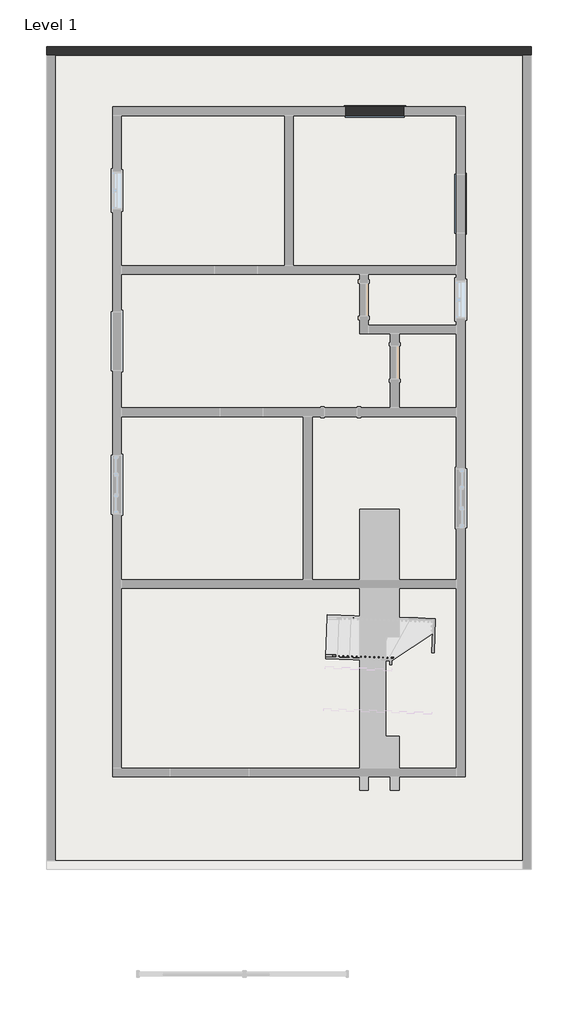
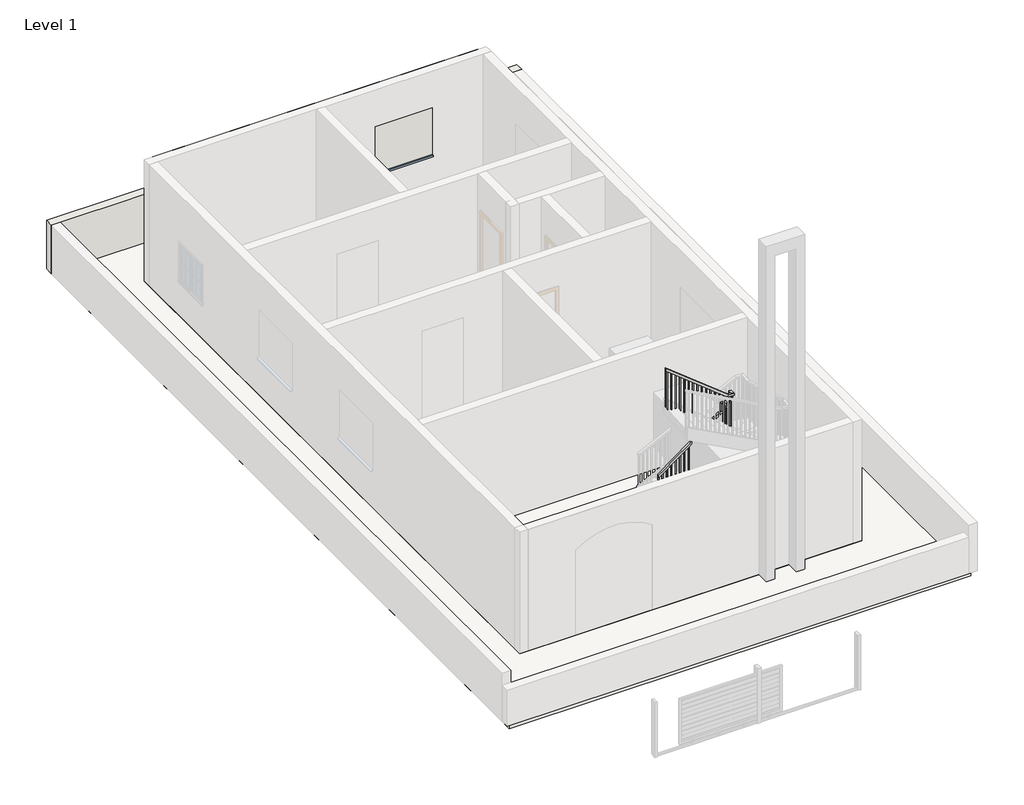
# One storey, part 2 of 4: 3 slabs, 2 railings, 2 walls, 2 windows.
"""IFC4 building model written with IfcOpenShell, lengths in millimetres."""

from ifc_helpers import new_model, si_unit, frame, origin, place, context, project, spatial, polyline, outline, extrude, faceted_brep, transform, mapped, element, save
from components import windows_tpl_plain_1360x1210mm_e2a6c9d8

model = new_model("IFC4")

# Units and contexts
model_context = context("Model", 3, world=origin())
ifc_project = project(units=[si_unit("LENGTHUNIT", "METRE", prefix="MILLI")], contexts=[model_context])

# Site, building, storey
site = spatial("IfcSite", under=ifc_project)
building = spatial("IfcBuilding", under=site)
storey = spatial("IfcBuildingStorey", under=building, Name="Level 1", Elevation=0.0)

# Railings
placement = place(None, origin())
element("IfcRailing", 1, ObjectType="Handrail - Rectangular", at=placement, inside=storey, context=model_context, shape_type="SolidModel", body=[
    faceted_brep([(-10037.4477622, -1226.3543786, 1083.7333333), (-10037.4477622, -1226.3543786, 1019.4000346), (-10039.2744432, -1277.1215258, 1019.4000346), (-10039.2744432, -1277.1215258, 1083.7333333), (-8586.854788, -1278.5489726, 2211.6191036), (-8536.0876408, -1280.3756536, 2186.7590024), (-8537.9143218, -1331.1428009, 2186.7590024), (-8588.681469, -1329.3161198, 2211.6191036), (-8586.854788, -1278.5489726, 2414.6281882), (-8536.0876408, -1280.3756536, 2363.8281882), (-8537.9143218, -1331.1428009, 2363.8281882), (-8588.681469, -1329.3161198, 2414.6281882), (-8459.9369199, -1283.1156752, 2414.6281882), (-8459.9369199, -1283.1156752, 2363.8281882), (-8512.5307482, -1332.0561414, 2363.8281882), (-8512.5307482, -1332.0561414, 2414.6281882), (-8464.5036225, -1410.0335432, 2414.6281882), (-8465.5507758, -1439.136044, 2363.8281882), (-8516.317923, -1437.309363, 2363.8281882), (-8515.2707697, -1408.2068622, 2414.6281882), (-8469.070325, -1536.9514112, 2631.5051451), (-8470.897006, -1587.7185585, 2617.7256424), (-8521.6641532, -1585.8918774, 2617.7256424), (-8519.8374722, -1535.1247302, 2631.5051451), (-8469.070325, -1536.9514112, 2834.5142297), (-8470.897006, -1587.7185585, 2783.7142297), (-8521.6641532, -1585.8918774, 2783.7142297), (-8519.8374722, -1535.1247302, 2834.5142297), (-8473.6370275, -1663.8692793, 2834.5142297), (-8473.6370275, -1663.8692793, 2783.7142297), (-8522.5774937, -1611.2754511, 2783.7142297), (-8522.5774937, -1611.2754511, 2834.5142297), (-8600.5548956, -1659.3025768, 2834.5142297), (-8617.9603, -1658.6763032, 2783.7142297), (-8616.133619, -1607.909156, 2783.7142297), (-8598.7282145, -1608.5354295, 2834.5142297), (-10051.1478698, -1607.1079827, 3962.4), (-10049.3211887, -1556.3408355, 3962.4), (-10049.3211887, -1556.3408355, 3898.0667013), (-10051.1478698, -1607.1079827, 3898.0667013)], [[[0, 1, 2, 3]], [[1, 0, 4, 5]], [[2, 1, 5, 6]], [[3, 2, 6, 7]], [[0, 3, 7, 4]], [[5, 4, 8, 9]], [[6, 5, 9, 10]], [[7, 6, 10, 11]], [[4, 7, 11, 8]], [[9, 8, 12, 13]], [[10, 9, 13, 14]], [[11, 10, 14, 15]], [[8, 11, 15, 12]], [[13, 12, 16, 17]], [[14, 13, 17, 18]], [[15, 14, 18, 19]], [[12, 15, 19, 16]], [[17, 16, 20, 21]], [[18, 17, 21, 22]], [[19, 18, 22, 23]], [[16, 19, 23, 20]], [[21, 20, 24, 25]], [[22, 21, 25, 26]], [[23, 22, 26, 27]], [[20, 23, 27, 24]], [[25, 24, 28, 29]], [[26, 25, 29, 30]], [[27, 26, 30, 31]], [[24, 27, 31, 28]], [[29, 28, 32, 33]], [[30, 29, 33, 34]], [[31, 30, 34, 35]], [[28, 31, 35, 32]], [[36, 37, 38, 39]], [[33, 32, 36, 39]], [[34, 33, 39, 38]], [[35, 34, 38, 37]], [[32, 35, 37, 36]]]),
    extrude(outline(polyline([(236.0012245, -19.05), (221.1987754, 0.0), (1225.3637939, 0.0), (1225.3637939, -19.05), (236.0012245, -19.05)])), frame((-10030.9830199, -1591.9482723, 4104.0304606), z_axis=(0.0359582876180528, 0.9993532916599503, 0.0), x_axis=(0.0, 0.0, -1.0)), (0.0, 0.0, 1.0), 19.05),
    extrude(outline(polyline([(236.0012246, -19.05), (221.1987755, 0.0), (1146.417399, 0.0), (1146.417399, -19.05), (236.0012246, -19.05)])), frame((-9929.4487255, -1595.6016343, 4025.0840657), z_axis=(0.0359582876180528, 0.9993532916599503, 0.0), x_axis=(0.0, 0.0, -1.0)), (0.0, 0.0, 1.0), 19.05),
    extrude(outline(polyline([(236.0012245, -19.05), (221.1987755, 0.0), (1067.471004, 0.0), (1067.471004, -19.05), (236.0012245, -19.05)])), frame((-9827.914431, -1599.2549963, 3946.1376707), z_axis=(0.0359582876180528, 0.9993532916599503, 0.0), x_axis=(0.0, 0.0, -1.0)), (0.0, 0.0, 1.0), 19.05),
    extrude(outline(polyline([(236.0012245, -19.05), (221.1987754, 0.0), (1157.8579424, 0.0), (1157.8579424, -19.05), (236.0012245, -19.05)])), frame((-9726.3801366, -1602.9083583, 3867.1912757), z_axis=(0.0359582876180528, 0.9993532916599503, 0.0), x_axis=(0.0, 0.0, -1.0)), (0.0, 0.0, 1.0), 19.05),
    extrude(outline(polyline([(236.0012246, -19.05), (221.1987755, 0.0), (1078.9115475, 0.0), (1078.9115475, -19.05), (236.0012246, -19.05)])), frame((-9624.8458422, -1606.5617203, 3788.2448808), z_axis=(0.0359582876180528, 0.9993532916599503, 0.0), x_axis=(0.0, 0.0, -1.0)), (0.0, 0.0, 1.0), 19.05),
    extrude(outline(polyline([(236.0012245, -19.05), (221.1987755, 0.0), (999.9651525, 0.0), (999.9651525, -19.05), (236.0012245, -19.05)])), frame((-9523.3115477, -1610.2150824, 3709.2984858), z_axis=(0.0359582876180528, 0.9993532916599503, 0.0), x_axis=(0.0, 0.0, -1.0)), (0.0, 0.0, 1.0), 19.05),
    extrude(outline(polyline([(236.0012245, -19.05), (221.1987754, 0.0), (1090.3520908, 0.0), (1090.3520908, -19.05), (236.0012245, -19.05)])), frame((-9421.7772533, -1613.8684444, 3630.3520908), z_axis=(0.0359582876180528, 0.9993532916599503, 0.0), x_axis=(0.0, 0.0, -1.0)), (0.0, 0.0, 1.0), 19.05),
    extrude(outline(polyline([(236.0012246, -19.05), (221.1987755, 0.0), (1011.4056959, 0.0), (1011.4056959, -19.05), (236.0012246, -19.05)])), frame((-9320.2429589, -1617.5218064, 3551.4056959), z_axis=(0.0359582876180528, 0.9993532916599503, 0.0), x_axis=(0.0, 0.0, -1.0)), (0.0, 0.0, 1.0), 19.05),
    extrude(outline(polyline([(236.0012245, -19.05), (221.1987755, 0.0), (1101.7926342, 0.0), (1101.7926342, -19.05), (236.0012245, -19.05)])), frame((-9218.7086644, -1621.1751684, 3472.4593009), z_axis=(0.0359582876180528, 0.9993532916599503, 0.0), x_axis=(0.0, 0.0, -1.0)), (0.0, 0.0, 1.0), 19.05),
    extrude(outline(polyline([(236.0012245, -19.05), (221.1987755, 0.0), (1022.8462392, 0.0), (1022.8462392, -19.05), (236.0012245, -19.05)])), frame((-9117.17437, -1624.8285304, 3393.5129059), z_axis=(0.0359582876180528, 0.9993532916599503, 0.0), x_axis=(0.0, 0.0, -1.0)), (0.0, 0.0, 1.0), 19.05),
    extrude(outline(polyline([(236.0012245, -19.05), (221.1987754, 0.0), (943.8998442, 0.0), (943.8998442, -19.05), (236.0012245, -19.05)])), frame((-9015.6400756, -1628.4818925, 3314.5665109), z_axis=(0.0359582876180528, 0.9993532916599503, 0.0), x_axis=(0.0, 0.0, -1.0)), (0.0, 0.0, 1.0), 19.05),
    extrude(outline(polyline([(236.0012246, -19.05), (221.1987755, 0.0), (1034.2867827, 0.0), (1034.2867827, -19.05), (236.0012246, -19.05)])), frame((-8914.1057811, -1632.1352545, 3235.620116), z_axis=(0.0359582876180528, 0.9993532916599503, 0.0), x_axis=(0.0, 0.0, -1.0)), (0.0, 0.0, 1.0), 19.05),
    extrude(outline(polyline([(236.0012245, -19.05), (221.1987755, 0.0), (955.3403877, 0.0), (955.3403877, -19.05), (236.0012245, -19.05)])), frame((-8812.5714867, -1635.7886165, 3156.673721), z_axis=(0.0359582876180528, 0.9993532916599503, 0.0), x_axis=(0.0, 0.0, -1.0)), (0.0, 0.0, 1.0), 19.05),
    extrude(outline(polyline([(236.0012245, -19.05), (221.1987754, 0.0), (1045.727326, 0.0), (1045.727326, -19.05), (236.0012245, -19.05)])), frame((-8711.0371923, -1639.4419785, 3077.727326), z_axis=(0.0359582876180528, 0.9993532916599503, 0.0), x_axis=(0.0, 0.0, -1.0)), (0.0, 0.0, 1.0), 19.05),
    extrude(outline(polyline([(236.0012246, -19.05), (221.1987755, 0.0), (966.7809311, 0.0), (966.7809311, -19.05), (236.0012246, -19.05)])), frame((-8609.5028978, -1643.0953406, 2998.7809311), z_axis=(0.0359582876180528, 0.9993532916599503, 0.0), x_axis=(0.0, 0.0, -1.0)), (0.0, 0.0, 1.0), 19.05),
    extrude(outline(polyline([(-8506.3702575, -1602.3274488), (-8487.3325773, -1603.0124541), (-8488.0175827, -1622.0501344), (-8507.0552629, -1621.365129), (-8506.3702575, -1602.3274488)])), frame((0.0, 0.0, 1693.3333333), z_axis=(0.0, 0.0, 1.0), x_axis=(1.0, 0.0, 0.0)), (0.0, 0.0, 1.0), 1090.3808964),
    extrude(outline(polyline([(244.8657718, -19.05), (212.3342282, 0.0), (1192.1994682, 0.0), (1192.1994682, -19.05), (244.8657718, -19.05)])), frame((-8484.3642207, -1520.5158399, 2716.1994682), z_axis=(-0.9993532916599502, 0.035958287618050686, 0.0), x_axis=(0.0, 0.0, -1.0)), (0.0, 0.0, 1.0), 19.05),
    extrude(outline(polyline([(244.8657717, -19.05), (212.3342282, 0.0), (1188.0312359, 0.0), (1188.0312359, -19.05), (244.8657717, -19.05)])), frame((-8480.7108586, -1418.9815455, 2542.6979026), z_axis=(-0.9993532916599502, 0.035958287618050686, 0.0), x_axis=(0.0, 0.0, -1.0)), (0.0, 0.0, 1.0), 19.05),
    extrude(outline(polyline([(-8525.208029, -1315.7147199), (-8524.5230236, -1296.6770397), (-8505.4853434, -1297.3620451), (-8506.1703488, -1316.3997253), (-8525.208029, -1315.7147199)])), frame((0.0, 0.0, 1185.3333333), z_axis=(0.0, 0.0, 1.0), x_axis=(1.0, 0.0, 0.0)), (0.0, 0.0, 1.0), 1178.4948549),
    extrude(outline(polyline([(221.1987754, -19.05), (236.0012245, 0.0), (1337.2495642, 0.0), (1337.2495642, -19.05), (221.1987754, -19.05)])), frame((-8626.7423234, -1312.0613579, 2353.2495642), z_axis=(0.035958287618052934, 0.9993532916599503, 0.0), x_axis=(0.0, 0.0, -1.0)), (0.0, 0.0, 1.0), 19.05),
    extrude(outline(polyline([(221.1987755, -19.0500001), (236.0012246, 0.0), (1258.3031693, 0.0), (1258.3031693, -19.0500001), (221.1987755, -19.0500001)])), frame((-8728.2766179, -1308.4079959, 2274.3031693), z_axis=(0.035958287618052934, 0.9993532916599503, 0.0), x_axis=(0.0, 0.0, -1.0)), (0.0, 0.0, 1.0), 19.05),
    extrude(outline(polyline([(221.1987755, -19.05), (236.0012245, 0.0), (1348.6901076, 0.0), (1348.6901076, -19.05), (221.1987755, -19.05)])), frame((-8829.8109123, -1304.7546339, 2195.3567743), z_axis=(0.035958287618052934, 0.9993532916599503, 0.0), x_axis=(0.0, 0.0, -1.0)), (0.0, 0.0, 1.0), 19.05),
    extrude(outline(polyline([(221.1987754, -19.05), (236.0012245, 0.0), (1269.7437126, 0.0), (1269.7437126, -19.05), (221.1987754, -19.05)])), frame((-8931.3452067, -1301.1012718, 2116.4103793), z_axis=(0.035958287618052934, 0.9993532916599503, 0.0), x_axis=(0.0, 0.0, -1.0)), (0.0, 0.0, 1.0), 19.05),
    extrude(outline(polyline([(221.1987755, -19.05), (236.0012246, 0.0), (1360.1306511, 0.0), (1360.1306511, -19.05), (221.1987755, -19.05)])), frame((-9032.8795011, -1297.4479098, 2037.4639844), z_axis=(0.035958287618052934, 0.9993532916599503, 0.0), x_axis=(0.0, 0.0, -1.0)), (0.0, 0.0, 1.0), 19.05),
    extrude(outline(polyline([(221.1987755, -19.05), (236.0012245, 0.0), (1281.1842561, 0.0), (1281.1842561, -19.05), (221.1987755, -19.05)])), frame((-9134.4137956, -1293.7945478, 1958.5175894), z_axis=(0.035958287618052934, 0.9993532916599503, 0.0), x_axis=(0.0, 0.0, -1.0)), (0.0, 0.0, 1.0), 19.05),
    extrude(outline(polyline([(221.1987755, -19.05), (236.0012245, 0.0), (1371.5711944, 0.0), (1371.5711944, -19.05), (221.1987755, -19.05)])), frame((-9235.94809, -1290.1411858, 1879.5711944), z_axis=(0.035958287618052934, 0.9993532916599503, 0.0), x_axis=(0.0, 0.0, -1.0)), (0.0, 0.0, 1.0), 19.05),
    extrude(outline(polyline([(221.1987754, -19.05), (236.0012245, 0.0), (1292.6247994, 0.0), (1292.6247994, -19.05), (221.1987754, -19.05)])), frame((-9337.4823844, -1286.4878237, 1800.6247994), z_axis=(0.035958287618052934, 0.9993532916599503, 0.0), x_axis=(0.0, 0.0, -1.0)), (0.0, 0.0, 1.0), 19.05),
    extrude(outline(polyline([(221.1987755, -19.05), (236.0012246, 0.0), (1213.6784045, 0.0), (1213.6784045, -19.05), (221.1987755, -19.05)])), frame((-9439.0166789, -1282.8344617, 1721.6784045), z_axis=(0.035958287618052934, 0.9993532916599503, 0.0), x_axis=(0.0, 0.0, -1.0)), (0.0, 0.0, 1.0), 19.05),
    extrude(outline(polyline([(221.1987755, -19.05), (236.0012245, 0.0), (1304.0653428, 0.0), (1304.0653428, -19.05), (221.1987755, -19.05)])), frame((-9540.5509733, -1279.1810997, 1642.7320095), z_axis=(0.035958287618052934, 0.9993532916599503, 0.0), x_axis=(0.0, 0.0, -1.0)), (0.0, 0.0, 1.0), 19.05),
    extrude(outline(polyline([(221.1987754, -19.05), (236.0012245, 0.0), (1225.1189478, 0.0), (1225.1189478, -19.05), (221.1987754, -19.05)])), frame((-9642.0852677, -1275.5277377, 1563.7856145), z_axis=(0.035958287618052934, 0.9993532916599503, 0.0), x_axis=(0.0, 0.0, -1.0)), (0.0, 0.0, 1.0), 19.05),
    extrude(outline(polyline([(221.1987755, -19.05), (236.0012246, 0.0), (1146.1725529, 0.0), (1146.1725529, -19.05), (221.1987755, -19.05)])), frame((-9743.6195622, -1271.8743757, 1484.8392196), z_axis=(0.035958287618052934, 0.9993532916599503, 0.0), x_axis=(0.0, 0.0, -1.0)), (0.0, 0.0, 1.0), 19.05),
    extrude(outline(polyline([(221.1987755, -19.05), (236.0012245, 0.0), (1236.5594913, 0.0), (1236.5594913, -19.05), (221.1987755, -19.05)])), frame((-9845.1538566, -1268.2210136, 1405.8928246), z_axis=(0.035958287618052934, 0.9993532916599503, 0.0), x_axis=(0.0, 0.0, -1.0)), (0.0, 0.0, 1.0), 19.05),
    extrude(outline(polyline([(221.1987755, -19.05), (236.0012245, 0.0), (1157.6130963, 0.0), (1157.6130963, -19.05), (221.1987755, -19.05)])), frame((-9946.688151, -1264.5676516, 1326.9464296), z_axis=(0.035958287618052934, 0.9993532916599503, 0.0), x_axis=(0.0, 0.0, -1.0)), (0.0, 0.0, 1.0), 19.05),
    extrude(outline(polyline([(-8507.283598, -1627.7110224), (-8488.2459178, -1628.3960278), (-8488.9309232, -1647.433708), (-8507.9686034, -1646.7487026), (-8507.283598, -1627.7110224)])), frame((0.0, 0.0, 1862.6666667), z_axis=(0.0, 0.0, 1.0), x_axis=(1.0, 0.0, 0.0)), (0.0, 0.0, 1.0), 921.0475631),
    extrude(outline(polyline([(-8496.0951768, -1316.7622457), (-8495.4101715, -1297.7245655), (-8476.3724912, -1298.4095708), (-8477.0574966, -1317.4472511), (-8496.0951768, -1316.7622457)])), frame((0.0, 0.0, 1185.3333333), z_axis=(0.0, 0.0, 1.0), x_axis=(1.0, 0.0, 0.0)), (0.0, 0.0, 1.0), 1178.4948549),
    extrude(outline(polyline([(236.0012245, -19.05), (221.1987755, 0.0), (1240.5988101, 0.0), (1240.5988101, -19.05), (236.0012245, -19.05)])), frame((-10050.5770319, -1591.2432492, 4119.2654768), z_axis=(0.0359582876180528, 0.9993532916599503, 0.0), x_axis=(0.0, 0.0, -1.0)), (0.0, 0.0, 1.0), 19.05),
    extrude(outline(polyline([(221.1987755, -19.05), (236.0012246, 0.0), (1086.0679259, 0.0), (1086.0679259, -19.05), (221.1987755, -19.05)])), frame((-10038.7036054, -1261.2567923, 1255.4012592), z_axis=(0.035958287618052934, 0.9993532916599503, 0.0), x_axis=(0.0, 0.0, -1.0)), (0.0, 0.0, 1.0), 19.05),
])
element("IfcRailing", 2, ObjectType="Handrail - Rectangular", at=placement, inside=storey, context=model_context, shape_type="SolidModel", body=[
    faceted_brep([(-10037.4477622, -1226.3543786, 1083.7333333), (-10037.4477622, -1226.3543786, 1019.4000346), (-10039.2744432, -1277.1215258, 1019.4000346), (-10039.2744432, -1277.1215258, 1083.7333333), (-8586.854788, -1278.5489726, 2211.6191036), (-8536.0876408, -1280.3756536, 2186.7590024), (-8537.9143218, -1331.1428009, 2186.7590024), (-8588.681469, -1329.3161198, 2211.6191036), (-8586.854788, -1278.5489726, 2414.6281882), (-8536.0876408, -1280.3756536, 2363.8281882), (-8537.9143218, -1331.1428009, 2363.8281882), (-8588.681469, -1329.3161198, 2414.6281882), (-8459.9369199, -1283.1156752, 2414.6281882), (-8459.9369199, -1283.1156752, 2363.8281882), (-8512.5307482, -1332.0561414, 2363.8281882), (-8512.5307482, -1332.0561414, 2414.6281882), (-8464.5036225, -1410.0335432, 2414.6281882), (-8465.5507758, -1439.136044, 2363.8281882), (-8516.317923, -1437.309363, 2363.8281882), (-8515.2707697, -1408.2068622, 2414.6281882), (-8469.070325, -1536.9514112, 2631.5051451), (-8470.897006, -1587.7185585, 2617.7256424), (-8521.6641532, -1585.8918774, 2617.7256424), (-8519.8374722, -1535.1247302, 2631.5051451), (-8469.070325, -1536.9514112, 2834.5142297), (-8470.897006, -1587.7185585, 2783.7142297), (-8521.6641532, -1585.8918774, 2783.7142297), (-8519.8374722, -1535.1247302, 2834.5142297), (-8473.6370275, -1663.8692793, 2834.5142297), (-8473.6370275, -1663.8692793, 2783.7142297), (-8522.5774937, -1611.2754511, 2783.7142297), (-8522.5774937, -1611.2754511, 2834.5142297), (-8600.5548956, -1659.3025768, 2834.5142297), (-8617.9603, -1658.6763032, 2783.7142297), (-8616.133619, -1607.909156, 2783.7142297), (-8598.7282145, -1608.5354295, 2834.5142297), (-10051.1478698, -1607.1079827, 3962.4), (-10049.3211887, -1556.3408355, 3962.4), (-10049.3211887, -1556.3408355, 3898.0667013), (-10051.1478698, -1607.1079827, 3898.0667013)], [[[0, 1, 2, 3]], [[1, 0, 4, 5]], [[2, 1, 5, 6]], [[3, 2, 6, 7]], [[0, 3, 7, 4]], [[5, 4, 8, 9]], [[6, 5, 9, 10]], [[7, 6, 10, 11]], [[4, 7, 11, 8]], [[9, 8, 12, 13]], [[10, 9, 13, 14]], [[11, 10, 14, 15]], [[8, 11, 15, 12]], [[13, 12, 16, 17]], [[14, 13, 17, 18]], [[15, 14, 18, 19]], [[12, 15, 19, 16]], [[17, 16, 20, 21]], [[18, 17, 21, 22]], [[19, 18, 22, 23]], [[16, 19, 23, 20]], [[21, 20, 24, 25]], [[22, 21, 25, 26]], [[23, 22, 26, 27]], [[20, 23, 27, 24]], [[25, 24, 28, 29]], [[26, 25, 29, 30]], [[27, 26, 30, 31]], [[24, 27, 31, 28]], [[29, 28, 32, 33]], [[30, 29, 33, 34]], [[31, 30, 34, 35]], [[28, 31, 35, 32]], [[36, 37, 38, 39]], [[33, 32, 36, 39]], [[34, 33, 39, 38]], [[35, 34, 38, 37]], [[32, 35, 37, 36]]]),
    extrude(outline(polyline([(236.0012245, -19.05), (221.1987754, 0.0), (1225.3637939, 0.0), (1225.3637939, -19.05), (236.0012245, -19.05)])), frame((-10030.9830199, -1591.9482723, 4104.0304606), z_axis=(0.0359582876180528, 0.9993532916599503, 0.0), x_axis=(0.0, 0.0, -1.0)), (0.0, 0.0, 1.0), 19.05),
    extrude(outline(polyline([(236.0012246, -19.05), (221.1987755, 0.0), (1146.417399, 0.0), (1146.417399, -19.05), (236.0012246, -19.05)])), frame((-9929.4487255, -1595.6016343, 4025.0840657), z_axis=(0.0359582876180528, 0.9993532916599503, 0.0), x_axis=(0.0, 0.0, -1.0)), (0.0, 0.0, 1.0), 19.05),
    extrude(outline(polyline([(236.0012245, -19.05), (221.1987755, 0.0), (1067.471004, 0.0), (1067.471004, -19.05), (236.0012245, -19.05)])), frame((-9827.914431, -1599.2549963, 3946.1376707), z_axis=(0.0359582876180528, 0.9993532916599503, 0.0), x_axis=(0.0, 0.0, -1.0)), (0.0, 0.0, 1.0), 19.05),
    extrude(outline(polyline([(236.0012245, -19.05), (221.1987754, 0.0), (1157.8579424, 0.0), (1157.8579424, -19.05), (236.0012245, -19.05)])), frame((-9726.3801366, -1602.9083583, 3867.1912757), z_axis=(0.0359582876180528, 0.9993532916599503, 0.0), x_axis=(0.0, 0.0, -1.0)), (0.0, 0.0, 1.0), 19.05),
    extrude(outline(polyline([(236.0012246, -19.05), (221.1987755, 0.0), (1078.9115475, 0.0), (1078.9115475, -19.05), (236.0012246, -19.05)])), frame((-9624.8458422, -1606.5617203, 3788.2448808), z_axis=(0.0359582876180528, 0.9993532916599503, 0.0), x_axis=(0.0, 0.0, -1.0)), (0.0, 0.0, 1.0), 19.05),
    extrude(outline(polyline([(236.0012245, -19.05), (221.1987755, 0.0), (999.9651525, 0.0), (999.9651525, -19.05), (236.0012245, -19.05)])), frame((-9523.3115477, -1610.2150824, 3709.2984858), z_axis=(0.0359582876180528, 0.9993532916599503, 0.0), x_axis=(0.0, 0.0, -1.0)), (0.0, 0.0, 1.0), 19.05),
    extrude(outline(polyline([(236.0012245, -19.05), (221.1987754, 0.0), (1090.3520908, 0.0), (1090.3520908, -19.05), (236.0012245, -19.05)])), frame((-9421.7772533, -1613.8684444, 3630.3520908), z_axis=(0.0359582876180528, 0.9993532916599503, 0.0), x_axis=(0.0, 0.0, -1.0)), (0.0, 0.0, 1.0), 19.05),
    extrude(outline(polyline([(236.0012246, -19.05), (221.1987755, 0.0), (1011.4056959, 0.0), (1011.4056959, -19.05), (236.0012246, -19.05)])), frame((-9320.2429589, -1617.5218064, 3551.4056959), z_axis=(0.0359582876180528, 0.9993532916599503, 0.0), x_axis=(0.0, 0.0, -1.0)), (0.0, 0.0, 1.0), 19.05),
    extrude(outline(polyline([(236.0012245, -19.05), (221.1987755, 0.0), (1101.7926342, 0.0), (1101.7926342, -19.05), (236.0012245, -19.05)])), frame((-9218.7086644, -1621.1751684, 3472.4593009), z_axis=(0.0359582876180528, 0.9993532916599503, 0.0), x_axis=(0.0, 0.0, -1.0)), (0.0, 0.0, 1.0), 19.05),
    extrude(outline(polyline([(236.0012245, -19.05), (221.1987755, 0.0), (1022.8462392, 0.0), (1022.8462392, -19.05), (236.0012245, -19.05)])), frame((-9117.17437, -1624.8285304, 3393.5129059), z_axis=(0.0359582876180528, 0.9993532916599503, 0.0), x_axis=(0.0, 0.0, -1.0)), (0.0, 0.0, 1.0), 19.05),
    extrude(outline(polyline([(236.0012245, -19.05), (221.1987754, 0.0), (943.8998442, 0.0), (943.8998442, -19.05), (236.0012245, -19.05)])), frame((-9015.6400756, -1628.4818925, 3314.5665109), z_axis=(0.0359582876180528, 0.9993532916599503, 0.0), x_axis=(0.0, 0.0, -1.0)), (0.0, 0.0, 1.0), 19.05),
    extrude(outline(polyline([(236.0012246, -19.05), (221.1987755, 0.0), (1034.2867827, 0.0), (1034.2867827, -19.05), (236.0012246, -19.05)])), frame((-8914.1057811, -1632.1352545, 3235.620116), z_axis=(0.0359582876180528, 0.9993532916599503, 0.0), x_axis=(0.0, 0.0, -1.0)), (0.0, 0.0, 1.0), 19.05),
    extrude(outline(polyline([(236.0012245, -19.05), (221.1987755, 0.0), (955.3403877, 0.0), (955.3403877, -19.05), (236.0012245, -19.05)])), frame((-8812.5714867, -1635.7886165, 3156.673721), z_axis=(0.0359582876180528, 0.9993532916599503, 0.0), x_axis=(0.0, 0.0, -1.0)), (0.0, 0.0, 1.0), 19.05),
    extrude(outline(polyline([(236.0012245, -19.05), (221.1987754, 0.0), (1045.727326, 0.0), (1045.727326, -19.05), (236.0012245, -19.05)])), frame((-8711.0371923, -1639.4419785, 3077.727326), z_axis=(0.0359582876180528, 0.9993532916599503, 0.0), x_axis=(0.0, 0.0, -1.0)), (0.0, 0.0, 1.0), 19.05),
    extrude(outline(polyline([(236.0012246, -19.05), (221.1987755, 0.0), (966.7809311, 0.0), (966.7809311, -19.05), (236.0012246, -19.05)])), frame((-8609.5028978, -1643.0953406, 2998.7809311), z_axis=(0.0359582876180528, 0.9993532916599503, 0.0), x_axis=(0.0, 0.0, -1.0)), (0.0, 0.0, 1.0), 19.05),
    extrude(outline(polyline([(-8506.3702575, -1602.3274488), (-8487.3325773, -1603.0124541), (-8488.0175827, -1622.0501344), (-8507.0552629, -1621.365129), (-8506.3702575, -1602.3274488)])), frame((0.0, 0.0, 1693.3333333), z_axis=(0.0, 0.0, 1.0), x_axis=(1.0, 0.0, 0.0)), (0.0, 0.0, 1.0), 1090.3808964),
    extrude(outline(polyline([(244.8657718, -19.05), (212.3342282, 0.0), (1192.1994682, 0.0), (1192.1994682, -19.05), (244.8657718, -19.05)])), frame((-8484.3642207, -1520.5158399, 2716.1994682), z_axis=(-0.9993532916599502, 0.035958287618050686, 0.0), x_axis=(0.0, 0.0, -1.0)), (0.0, 0.0, 1.0), 19.05),
    extrude(outline(polyline([(244.8657717, -19.05), (212.3342282, 0.0), (1188.0312359, 0.0), (1188.0312359, -19.05), (244.8657717, -19.05)])), frame((-8480.7108586, -1418.9815455, 2542.6979026), z_axis=(-0.9993532916599502, 0.035958287618050686, 0.0), x_axis=(0.0, 0.0, -1.0)), (0.0, 0.0, 1.0), 19.05),
    extrude(outline(polyline([(-8525.208029, -1315.7147199), (-8524.5230236, -1296.6770397), (-8505.4853434, -1297.3620451), (-8506.1703488, -1316.3997253), (-8525.208029, -1315.7147199)])), frame((0.0, 0.0, 1185.3333333), z_axis=(0.0, 0.0, 1.0), x_axis=(1.0, 0.0, 0.0)), (0.0, 0.0, 1.0), 1178.4948549),
    extrude(outline(polyline([(221.1987754, -19.05), (236.0012245, 0.0), (1337.2495642, 0.0), (1337.2495642, -19.05), (221.1987754, -19.05)])), frame((-8626.7423234, -1312.0613579, 2353.2495642), z_axis=(0.035958287618052934, 0.9993532916599503, 0.0), x_axis=(0.0, 0.0, -1.0)), (0.0, 0.0, 1.0), 19.05),
    extrude(outline(polyline([(221.1987755, -19.0500001), (236.0012246, 0.0), (1258.3031693, 0.0), (1258.3031693, -19.0500001), (221.1987755, -19.0500001)])), frame((-8728.2766179, -1308.4079959, 2274.3031693), z_axis=(0.035958287618052934, 0.9993532916599503, 0.0), x_axis=(0.0, 0.0, -1.0)), (0.0, 0.0, 1.0), 19.05),
    extrude(outline(polyline([(221.1987755, -19.05), (236.0012245, 0.0), (1348.6901076, 0.0), (1348.6901076, -19.05), (221.1987755, -19.05)])), frame((-8829.8109123, -1304.7546339, 2195.3567743), z_axis=(0.035958287618052934, 0.9993532916599503, 0.0), x_axis=(0.0, 0.0, -1.0)), (0.0, 0.0, 1.0), 19.05),
    extrude(outline(polyline([(221.1987754, -19.05), (236.0012245, 0.0), (1269.7437126, 0.0), (1269.7437126, -19.05), (221.1987754, -19.05)])), frame((-8931.3452067, -1301.1012718, 2116.4103793), z_axis=(0.035958287618052934, 0.9993532916599503, 0.0), x_axis=(0.0, 0.0, -1.0)), (0.0, 0.0, 1.0), 19.05),
    extrude(outline(polyline([(221.1987755, -19.05), (236.0012246, 0.0), (1360.1306511, 0.0), (1360.1306511, -19.05), (221.1987755, -19.05)])), frame((-9032.8795011, -1297.4479098, 2037.4639844), z_axis=(0.035958287618052934, 0.9993532916599503, 0.0), x_axis=(0.0, 0.0, -1.0)), (0.0, 0.0, 1.0), 19.05),
    extrude(outline(polyline([(221.1987755, -19.05), (236.0012245, 0.0), (1281.1842561, 0.0), (1281.1842561, -19.05), (221.1987755, -19.05)])), frame((-9134.4137956, -1293.7945478, 1958.5175894), z_axis=(0.035958287618052934, 0.9993532916599503, 0.0), x_axis=(0.0, 0.0, -1.0)), (0.0, 0.0, 1.0), 19.05),
    extrude(outline(polyline([(221.1987755, -19.05), (236.0012245, 0.0), (1371.5711944, 0.0), (1371.5711944, -19.05), (221.1987755, -19.05)])), frame((-9235.94809, -1290.1411858, 1879.5711944), z_axis=(0.035958287618052934, 0.9993532916599503, 0.0), x_axis=(0.0, 0.0, -1.0)), (0.0, 0.0, 1.0), 19.05),
    extrude(outline(polyline([(221.1987754, -19.05), (236.0012245, 0.0), (1292.6247994, 0.0), (1292.6247994, -19.05), (221.1987754, -19.05)])), frame((-9337.4823844, -1286.4878237, 1800.6247994), z_axis=(0.035958287618052934, 0.9993532916599503, 0.0), x_axis=(0.0, 0.0, -1.0)), (0.0, 0.0, 1.0), 19.05),
    extrude(outline(polyline([(221.1987755, -19.05), (236.0012246, 0.0), (1213.6784045, 0.0), (1213.6784045, -19.05), (221.1987755, -19.05)])), frame((-9439.0166789, -1282.8344617, 1721.6784045), z_axis=(0.035958287618052934, 0.9993532916599503, 0.0), x_axis=(0.0, 0.0, -1.0)), (0.0, 0.0, 1.0), 19.05),
    extrude(outline(polyline([(221.1987755, -19.05), (236.0012245, 0.0), (1304.0653428, 0.0), (1304.0653428, -19.05), (221.1987755, -19.05)])), frame((-9540.5509733, -1279.1810997, 1642.7320095), z_axis=(0.035958287618052934, 0.9993532916599503, 0.0), x_axis=(0.0, 0.0, -1.0)), (0.0, 0.0, 1.0), 19.05),
    extrude(outline(polyline([(221.1987754, -19.05), (236.0012245, 0.0), (1225.1189478, 0.0), (1225.1189478, -19.05), (221.1987754, -19.05)])), frame((-9642.0852677, -1275.5277377, 1563.7856145), z_axis=(0.035958287618052934, 0.9993532916599503, 0.0), x_axis=(0.0, 0.0, -1.0)), (0.0, 0.0, 1.0), 19.05),
    extrude(outline(polyline([(221.1987755, -19.05), (236.0012246, 0.0), (1146.1725529, 0.0), (1146.1725529, -19.05), (221.1987755, -19.05)])), frame((-9743.6195622, -1271.8743757, 1484.8392196), z_axis=(0.035958287618052934, 0.9993532916599503, 0.0), x_axis=(0.0, 0.0, -1.0)), (0.0, 0.0, 1.0), 19.05),
    extrude(outline(polyline([(221.1987755, -19.05), (236.0012245, 0.0), (1236.5594913, 0.0), (1236.5594913, -19.05), (221.1987755, -19.05)])), frame((-9845.1538566, -1268.2210136, 1405.8928246), z_axis=(0.035958287618052934, 0.9993532916599503, 0.0), x_axis=(0.0, 0.0, -1.0)), (0.0, 0.0, 1.0), 19.05),
    extrude(outline(polyline([(221.1987755, -19.05), (236.0012245, 0.0), (1157.6130963, 0.0), (1157.6130963, -19.05), (221.1987755, -19.05)])), frame((-9946.688151, -1264.5676516, 1326.9464296), z_axis=(0.035958287618052934, 0.9993532916599503, 0.0), x_axis=(0.0, 0.0, -1.0)), (0.0, 0.0, 1.0), 19.05),
    extrude(outline(polyline([(-8507.283598, -1627.7110224), (-8488.2459178, -1628.3960278), (-8488.9309232, -1647.433708), (-8507.9686034, -1646.7487026), (-8507.283598, -1627.7110224)])), frame((0.0, 0.0, 1862.6666667), z_axis=(0.0, 0.0, 1.0), x_axis=(1.0, 0.0, 0.0)), (0.0, 0.0, 1.0), 921.0475631),
    extrude(outline(polyline([(-8496.0951768, -1316.7622457), (-8495.4101715, -1297.7245655), (-8476.3724912, -1298.4095708), (-8477.0574966, -1317.4472511), (-8496.0951768, -1316.7622457)])), frame((0.0, 0.0, 1185.3333333), z_axis=(0.0, 0.0, 1.0), x_axis=(1.0, 0.0, 0.0)), (0.0, 0.0, 1.0), 1178.4948549),
    extrude(outline(polyline([(236.0012245, -19.05), (221.1987755, 0.0), (1240.5988101, 0.0), (1240.5988101, -19.05), (236.0012245, -19.05)])), frame((-10050.5770319, -1591.2432492, 4119.2654768), z_axis=(0.0359582876180528, 0.9993532916599503, 0.0), x_axis=(0.0, 0.0, -1.0)), (0.0, 0.0, 1.0), 19.05),
    extrude(outline(polyline([(221.1987755, -19.05), (236.0012246, 0.0), (1086.0679259, 0.0), (1086.0679259, -19.05), (221.1987755, -19.05)])), frame((-10038.7036054, -1261.2567923, 1255.4012592), z_axis=(0.035958287618052934, 0.9993532916599503, 0.0), x_axis=(0.0, 0.0, -1.0)), (0.0, 0.0, 1.0), 19.05),
])

# Slabs
element("IfcSlab", 3, ObjectType="Generic - 12\"", at=placement, inside=storey, context=model_context, shape_type="SweptSolid", body=[
    extrude(outline(polyline([(-6821.5126504, 11392.728857), (-6821.5126504, -4050.471143), (-14949.5126504, -4050.471143), (-14949.5126504, 11392.728857), (-6821.5126504, 11392.728857)])), frame((0.0, 0.0, -152.4), z_axis=(0.0, 0.0, 1.0), x_axis=(1.0, 0.0, 0.0)), (0.0, 0.0, 1.0), 152.4),
])
element("IfcSlab", 4, ObjectType="Generic - 12\"", at=placement, inside=storey, context=model_context, shape_type="SweptSolid", body=[
    extrude(outline(polyline([(-6821.5126504, 11392.728857), (-6821.5126504, -4050.471143), (-14949.5126504, -4050.471143), (-14949.5126504, 11392.728857), (-6821.5126504, 11392.728857)])), frame((0.0, 0.0, -152.4), z_axis=(0.0, 0.0, 1.0), x_axis=(1.0, 0.0, 0.0)), (0.0, 0.0, 1.0), 152.4),
])
element("IfcSlab", 5, ObjectType="Generic - 12\"", at=placement, inside=storey, context=model_context, shape_type="SweptSolid", body=[
    extrude(outline(polyline([(-5399.1126504, 12681.3156917), (-5399.1126504, -6082.471143), (-16371.9126504, -6082.471143), (-16371.9126504, 12681.3156917), (-5399.1126504, 12681.3156917)])), frame((0.0, 0.0, -152.4), z_axis=(0.0, 0.0, 1.0), x_axis=(1.0, 0.0, 0.0)), (0.0, 0.0, 1.0), 152.4),
])

# Walls
element("IfcWall", 6, ObjectType="Generic - 4.5\" p", at=placement, inside=storey, context=model_context, shape_type="Brep", body=[
    faceted_brep([(-16473.5126504, 12579.7156917, 0.0), (-16270.3126504, 12579.7156917, 0.0), (-5500.7126504, 12579.7156917, 0.0), (-5297.5126504, 12579.7156917, 0.0), (-5297.5126504, 12579.7156917, 1219.2), (-5500.7126504, 12579.7156917, 1219.2), (-16270.3126504, 12579.7156917, 1219.2), (-16473.5126504, 12579.7156917, 1219.2), (-16473.5126504, 12782.9156917, 0.0), (-16473.5126504, 12782.9156917, 1219.2), (-5297.5126504, 12782.9156917, 1219.2), (-5297.5126504, 12782.9156917, 0.0)], [[[0, 1, 2, 3, 4, 5, 6, 7]], [[8, 9, 10, 11]], [[3, 2, 1, 0, 8, 11]], [[7, 6, 5, 4, 10, 9]], [[4, 3, 11, 10]], [[0, 7, 9, 8]]]),
])
element("IfcWall", 7, ObjectType="Generic - 9\" w", at=placement, inside=storey, context=model_context, shape_type="Brep", body=[
    faceted_brep([(-14746.3126504, 11189.528857, 0.0), (-10987.1126504, 11189.528857, 0.0), (-10783.9126504, 11189.528857, 0.0), (-7024.7126504, 11189.528857, 0.0), (-7024.7126504, 11189.528857, 3048.0), (-10783.9126504, 11189.528857, 3048.0), (-10987.1126504, 11189.528857, 3048.0), (-14746.3126504, 11189.528857, 3048.0), (-14746.3126504, 11392.728857, 0.0), (-14746.3126504, 11392.728857, 3048.0), (-7024.7126504, 11392.728857, 3048.0), (-7024.7126504, 11392.728857, 0.0)], [[[0, 1, 2, 3, 4, 5, 6, 7]], [[8, 9, 10, 11]], [[3, 2, 1, 0, 8, 11]], [[7, 6, 5, 4, 10, 9]], [[0, 7, 9, 8]], [[4, 3, 11, 10]]]),
])

# Windows
windows_tpl_plain_1360x1210mm_shape = windows_tpl_plain_1360x1210mm_e2a6c9d8(model_context)
element("IfcWindow", 8, ObjectType="Windows_Tpl_Plain : 1360x1210mm", at=placement, inside=storey, context=model_context, shape_type="MappedRepresentation", body=[
    mapped(windows_tpl_plain_1360x1210mm_shape, transform((-9405.979317, 11299.5854248, 14.4), x_axis=(-1.0, 0.0, 0.0), y_axis=(0.0, -1.0, 0.0), z_axis=(0.0, 0.0, 1.0))),
])
element("IfcWindow", 9, ObjectType="Windows_Tpl_Plain : 1360x1210mm", at=placement, inside=storey, context=model_context, shape_type="MappedRepresentation", body=[
    mapped(windows_tpl_plain_1360x1210mm_shape, transform((-6914.6560825, 9659.1955236, 14.4), x_axis=(0.0, 1.0, 0.0), y_axis=(-1.0, 0.0, 0.0), z_axis=(0.0, 0.0, 1.0))),
])

save(model, "model.ifc")

# Revit data of these elements
# Type "Handrail - Rectangular"
#   Assembly Code = "C2010400"
#   built-in parameter 1008612 = 0.0416667 (stored number, unit not read)
#   built-in parameter 1008611 = 0.0416667 (stored number, unit not read)
#   built-in parameter 1008609 = 0.333333 (stored number, unit not read)
#   built-in parameter 1008604 = 0.166667 (stored number, unit not read)
#   built-in parameter 1008603 = 0.166667 (stored number, unit not read)
#   Railing Height = 3' - 0"
#   built-in parameter 1008630 = 2
#   built-in parameter 1008610 = 2
#   built-in parameter 1008618 = Baluster - Square : 3/4"
# Type "Generic - 12\""
#   Assembly Code = "B1010"
#   Function = 0
#   Layers, outside or top first: 0' - 6" no material (function 1)
# Type "Generic - 4.5\" p"
#   Assembly Code = "B2010"
#   Layers, outside or top first: 0' - 8" "Brick, Common" (function 1)
# Type "Generic - 9\" w"
#   Assembly Code = "B2010"
#   Layers, outside or top first: 0' - 8" no material (function 1)
# Type "Windows_Tpl_Plain : 1360x1210mm"
#   Type Mark = "21"
#   Operation = "TriplePanelVertical"
#   Construction Type Id = "GSP4R"
#   Manufacturer = "Revit"
#   Keynote = "L10"
#   Analytic Construction = "1/8 in Pilkington single glazing"
#   Wrap Layers (Ext) from Ext = 0' - 4.03543"
#   Wrap Layers (Int) from Ext = 0' - 6.98819"
#   Window Board Projection = 0' - 0.98425"
#   Window Board Extension = 0' - 0.98425"
#   Visual Light Transmittance = 0.9
#   Solar Heat Gain Coefficient = 0.78
#   Rough Width = 4' - 5.54331"
#   Rough Height = 3' - 11.6378"
#   Height = 3' - 11.6378"
#   Width = 4' - 5.54331"
#   Heat Transfer Coefficient (U) = 0.6496 BTU/(h·ft²·°F)
#   Glazing Thickness = 0' - 0.94488"
#   FrameOffset - External = 0' - 1.9685"
#   Frame Depth = 0' - 2.55906"
#   Default Head Height = 6' - 11.07087"
#   Cill Depth = 0' - 3.44488"
#   Cavity Closer Width = 0' - 1.9685"
#   Cavity Closer Offset from Ext = 0' - 4.03543"
#   Cavity Closer Depth = 0' - 3.34646"
#   Vis - Cavity Closers = yes
#   Define Thermal Properties by = 1
#   Material Trim = Window Frame
#   Material Glass = Glass
#   Material Frame = Window Frame
#   Wall Closure = (empty or 0)
# Elements 1, 2 (IfcRailing, "Handrail - Rectangular")
#   Phase Created = New Construction
# Elements 3, 4 (IfcSlab, "Generic - 12\"")
#   Height Offset From Level = 0' - 0"
#   Phase Created = New Construction
#   Materials on its faces: "Default Floor", "Brick, Common"
# Element 5 (IfcSlab, "Generic - 12\"")
#   Height Offset From Level = 0' - 0"
#   Phase Created = New Construction
#   Materials on its faces: "Default Floor", "Brick, Soldier Course"
# Element 6 (IfcWall, "Generic - 4.5\" p")
#   Top Offset = 0' - 0"
#   Base Offset = 0' - 0"
#   Unconnected Height = 4' - 0"
#   wall height = 4' - 0"
#   Phase Created = New Construction
#   Base Constraint = Level 1
#   Materials on its faces: "Brick, Common", "Aluminum"
# Element 7 (IfcWall, "Generic - 9\" w")
#   Top Offset = 0' - 0"
#   Base Offset = 0' - 0"
#   wall height = 10' - 0"
#   Phase Created = New Construction
#   Base Constraint = Level 1
#   Top Constraint = Level 2
#   Materials on its faces: "Default Wall", "Cherry"
# Element 8 (IfcWindow, "Windows_Tpl_Plain : 1360x1210mm")
#   Mark = "1"
#   Phase Created = New Construction
#   Materials on its faces: "Window Frame", "Glass"
# Element 9 (IfcWindow, "Windows_Tpl_Plain : 1360x1210mm")
#   Mark = "2"
#   Phase Created = New Construction
#   Materials on its faces: "Window Frame", "Glass"
# Materials
#   "Brick, Common": class "Masonry", colour RGB 128 0 128, transparency 0, Description = "Common brick", Cost = 0
#   "Window Frame": colour RGB 249 249 249, transparency 0
#   "Glass": class "Glass", colour RGB 0 128 192, transparency 0.75, Description = "Soda Lime Glass", Cost = 0
#   "Default Floor": colour RGB 128 128 128, transparency 0, Cost = 0
#   "Brick, Soldier Course": class "Masonry", colour RGB 170 98 104, transparency 0, Description = "Common brick soldier coursed", Cost = 0
#   "Aluminum": class "Metal", colour RGB 247 247 247, transparency 0, Description = "Aluminum 6061", Cost = 0
#   "Default Wall": colour RGB 128 128 128, transparency 0, Cost = 0
#   "Cherry": class "Wood", colour RGB 226 177 128, transparency 0, Description = "Prunus Serotina", Cost = 0
